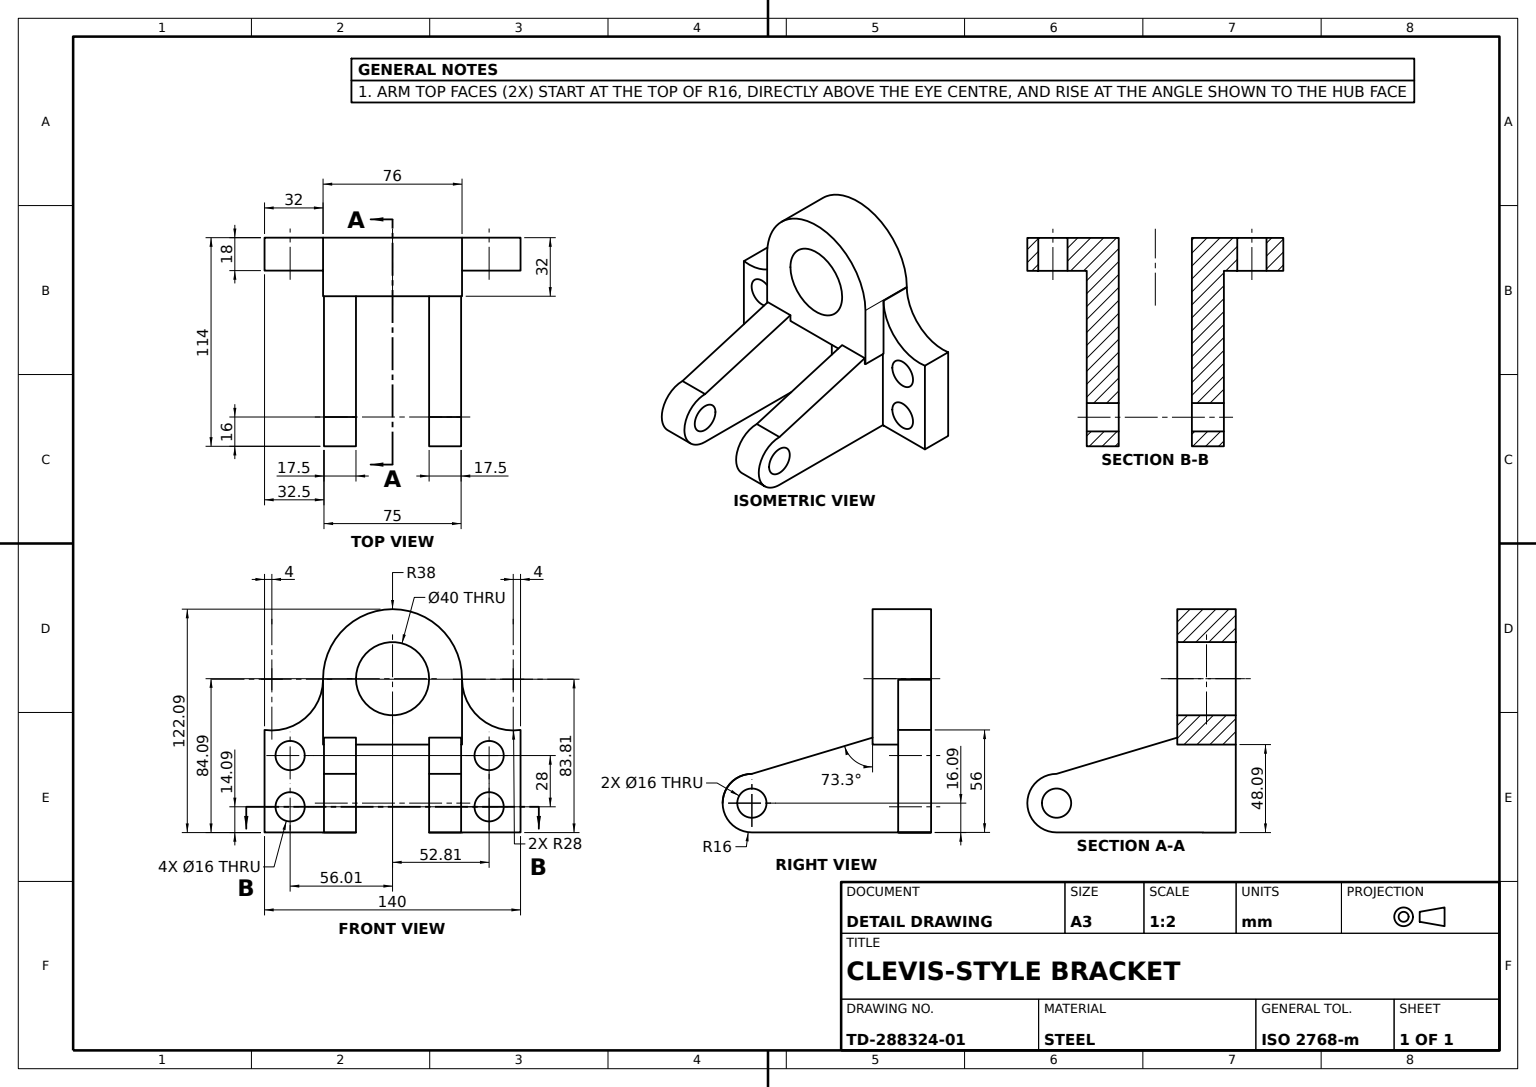
SolidWorks part; units mm, degrees
material "Plain Carbon Steel"
ref_plane "Front Plane" through (0, 0, 0) normal (0, 0, 1) x (1, 0, 0)
ref_plane "Top Plane" through (0, 0, 0) normal (0, 1, 0) x (1, 0, 0)
ref_plane "Right Plane" through (0, 0, 0) normal (1, 0, 0) x (0, 0, -1)
sketch "Hub Body Sketch" plane through (0, 0, 0) normal (0, 0, 1) x (1, 0, 0)
  line L0 (0, 0) -> (0, 49.2348) construction
  line L1 (0, 49.2348) -> (0, -56.0182) construction
  line L2 (0, -56.0182) -> (0, 0) construction
  line L3 (0, 0) -> (-83.2615, 0) construction
  line L4 (-83.2615, 0) -> (78.4474, 0) construction
  line L5 (-38, 36) -> (-38, 0)
  line L6 (-38, 0) -> (38, 0)
  line L7 (38, 0) -> (38, 36)
  arc A0 (38, 36) -> (-38, 36) centre (0, 36) ccw
  circle A1 centre (0, 36) radius 20
  dimension "D1" = 76
  dimension "D2" = 40
  dimension "D3" = 36
  dimension "D4" = 49.2348
  dimension "D5" = 56.0182
  dimension "D6" = 83.2615
extrude "Hub Body" add sketch "Hub Body Sketch" along normal blind 32
sketch "Mounting Plate Sketch" plane through (0, 0, 0) normal (0, 0, 1) x (1, 0, 0)
  line L0 (-38, 36) -> (-38, -48)
  line L1 (-38, -48) -> (-70, -48)
  line L2 (-70, -48) -> (-70, 8)
  line L3 (0, 0) -> (0, -68.4021)
  line L4 (38, 36) -> (38, -48)
  line L5 (38, -48) -> (70, -48)
  line L6 (70, -48) -> (70, 8)
  arc A0 (-70, 8) -> (-38, 36) centre (-65.9985, 35.7126) ccw
  arc A1 (70, 8) -> (38, 36) centre (65.9985, 35.7126) cw
  dimension "D4" = 28
  dimension "D1" = 84
  dimension "D2" = 32
  dimension "D3" = 56
  dimension "D5" = 20.4021
extrude "Mounting Plate" add sketch "Mounting Plate Sketch" along normal blind 18 contours A0 L2 L1 L0 | L6 A1 L4 L5
sketch "Side Web Sketch" plane through (0, 0, 0) normal (0, 0, 1) x (1, 0, 0)
  line L1 (-38, 0) -> (-20, 0)
  line L2 (-38, 0) -> (-38, -48.0929)
  line L3 (-38, -48.0929) -> (-20, -48.0929)
  line L4 (-20, 0) -> (-20, -48.0929)
  line L5 (38, 0) -> (20, 0)
  line L6 (38, 0) -> (38, -48.0929)
  line L7 (38, -48.0929) -> (20, -48.0929)
  line L8 (20, 0) -> (20, -48.0929)
  dimension "D1" = 18
  dimension "D2" = 18
  dimension "D3" = 48.0929
extrude "Side Web" add sketch "Side Web Sketch" along normal blind 18
sketch "Fork Arms Sketch" plane through (0, 0, 0) normal (1, 0, 0) x (0, 0, -1)
  line L0 (-18, -48) -> (-98, -48)
  line L1 (-18, 8) -> (-18, -48)
  line L2 (-98, -16) -> (-18, 8)
  circle A0 centre (-98, -32) radius 8
  circle A1 centre (-98, -32) radius 16
  dimension "D3" = 16
  dimension "D1" = 80
  dimension "D2" = 32
extrude "Fork Arms" add sketch "Fork Arms Sketch" along normal mid plane 75 contours A1 L0 L1 L2
sketch "Fork Slot Sketch" plane through (0, 0, 18) normal (0, 0, -1) x (-1, 0, 0)
  line L1 (-20, 0) -> (20, 0)
  line L2 (-20, 0) -> (-20, -48)
  line L3 (-20, -48) -> (20, -48)
  line L4 (20, 0) -> (20, -48)
extrude "Fork Slot" cut sketch "Fork Slot Sketch" against normal through all
sketch "Hub Relief Sketch" plane through (0, 0, 0) normal (0, -1, 0) x (-1, 0, 0)
  line L0 (-20, -44.6667) -> (20, -44.6667) construction
  line L1 (20, -44.6667) -> (-20, -44.6667)
  line L2 (20, -44.6667) -> (20, -18)
  line L3 (20, -18) -> (-20, -18)
  line L4 (-20, -44.6667) -> (-20, -18)
  line L5 (20, -44.6667) -> (20, 0) construction
  line L6 (11.0784, -32) -> (-20, -32)
  line L7 (11.0784, -32) -> (20, -32)
  line L8 (-20, -44.6667) -> (-20, 0) construction
  line M6 (-20, -44.6667) -> (20, -44.6667)
  line M7 (20, -44.6667) -> (20, 0)
  dimension "D1" = 31.0784
  dimension "D2" = 32
extrude "Hub Relief Cut" cut sketch "Hub Relief Sketch" against normal through all contours L7 L6 L4 M6 M7
sketch "Fork Pin Hole Sketch" plane through (-37.5, 0, 0) normal (-1, 0, 0) x (0, 0, 1)
  circle A0 centre (98, -32) radius 8
  dimension "D1" = 16
extrude "Fork Pin Hole Ø16" cut sketch "Fork Pin Hole Sketch" against normal through all contours A0
sketch "Plate Mounting Holes Sketch" plane through (0, 0, 18) normal (0, 0, 1) x (1, 0, 0)
  circle A0 centre (-56.0065, -6) radius 8
  circle A1 centre (-56.0065, -34) radius 8
  circle A2 centre (52.8126, -6) radius 8
  circle A3 centre (52.8126, -34) radius 8
  dimension "D1" = 16
  dimension "D2" = 14
  dimension "D3" = 14
  dimension "D4" = 28
  dimension "D5" = 28
  dimension "D6" = 56.0065
  dimension "D7" = 52.8126
extrude "Plate Mounting Holes Ø16" cut sketch "Plate Mounting Holes Sketch" against normal through all
